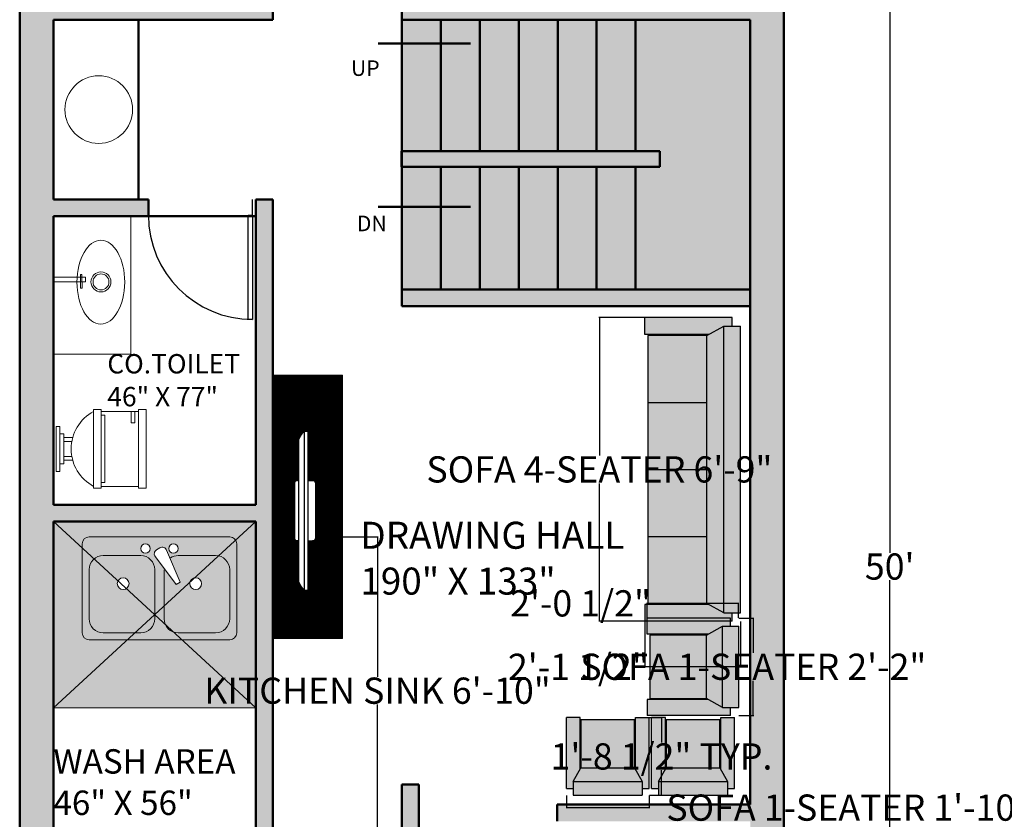
# Model space of a CAD drawing. Units: inches. Extents: x 679 to 1269, y 101 to 755.
# Tile 3 of 6: x 708 to 971, y 370 to 584. Entities that reach past the tile are written whole.
import ezdxf

# ---------------------------------------------------------------- set-up
doc = ezdxf.new("R2010")
doc.units = ezdxf.units.IN
doc.header["$MEASUREMENT"] = 0
for name, color, linetype, lineweight in [('A-ANNO-DIMS', 2, 'Continuous', 18), ('A-ANNO-TEXT', 7, 'Continuous', 25), ('A-AREA-IDEN', 7, 'Continuous', 25), ('A-DOOR', 4, 'Continuous', 25), ('A-FLOR-FIXT', 8, 'Continuous', 18), ('A-FLOR-PATT', 8, 'Continuous', 13), ('A-FURN', 32, 'Continuous', 18), ('A-FURN-PATT', 252, 'Continuous', 13), ('A-WALL', 7, 'Continuous', 50), ('A-WALL-PATT', 8, 'Continuous', 13)]:
    doc.layers.add(name, color=color, linetype=linetype, lineweight=lineweight)
doc.layers.add('furniture', color=32, linetype='Continuous')
doc.styles.add('ATT', font='TXT')
doc.styles.get("Standard").update_dxf_attribs({"font": 'arial.ttf'})
doc.dimstyles.get("Standard").update_dxf_attribs({"dimtxt": 7, "dimasz": 0.18, "dimexe": 0.18, "dimexo": 0.0625, "dimgap": 0.09, "dimtad": 0, "dimtih": 1, "dimtoh": 1, "dimzin": 0, "dimdsep": 46, "dimlunit": 3, "dimtxsty": 'Standard', "dimcen": 0.09, "dimadec": 0, "dimazin": 0, "dimtfac": 1, "dimtofl": 0, "dimtmove": 0, "dimatfit": 3, "dimfxl": 1, "dimtolj": 1, "dimtzin": 0, "dimarcsym": 0})

# ---------------------------------------------------------------- blocks, each defined once
blk = doc.blocks.new('*D2')
at = {"layer": 'A-ANNO-DIMS', "color": 0, "lineweight": -2, "transparency": 16777216}
for p, q in [((939.65, 737.73), (940.62, 737.73)), ((940.44, 737.55), (940.44, 441.39)), ((940.44, 137.91), (940.44, 434.07)), ((939.65, 137.73), (940.62, 137.73))]:
    blk.add_line(p, q, dxfattribs=at)
at = {"layer": 'A-ANNO-DIMS', "color": 0, "transparency": 16777216}
for points in [[(940.41, 737.55), (940.47, 737.55), (940.44, 737.73)], [(940.41, 137.91), (940.47, 137.91), (940.44, 137.73)]]:
    blk.add_solid(points, dxfattribs=at)
at = {"layer": 'Defpoints', "color": 0, "transparency": 16777216}
for p in [(939.59, 737.73), (939.59, 137.73), (940.44, 137.73)]:
    blk.add_point(p, dxfattribs=at)
at = {"layer": 'A-ANNO-DIMS', "color": 0, "transparency": 16777216, "insert": (940.44, 437.73), "char_height": 7, "attachment_point": 5}
blk.add_mtext("\\A1;50'", dxfattribs=at)
blk = doc.blocks.new('*U4')
for p, q in [((0, 0), (0, -6)), ((40, 0), (40, -6))]:
    blk.add_line(p, q)
blk.add_lwpolyline([(0, 0), (0, 40), (1.75, 40), (1.75, 0)], close=True)
blk.add_arc((0, 0), 40, 0, 90)
blk = doc.blocks.new('15PSNK10')
at = {"color": 0, "linetype": 'ByBlock'}
for p, q in [((0, 15), (0, -15)), ((20.5, 16.5), (1.5, 16.5)), ((7, 15), (17.5, 15)), ((22, -15), (22, 15)), ((4, 4), (4, 12)), ((20.5, 12), (20.5, 4)), ((2.37, -0.1), (2.77, 0.6)), ((10.18, -3.57), (4.27, 0.87)), ((17.5, 1), (7, 1)), ((2.88, -1.54), (9.68, -4.43)), ((7.04, -1), (17.5, -1)), ((4, -12), (4, -4)), ((9.68, -4.43), (10.18, -3.57)), ((20.5, -4), (20.5, -12)), ((1.5, -16.5), (20.5, -16.5)), ((17.5, -15), (7, -15))]:
    blk.add_line(p, q, dxfattribs=at)
for centre, radius in [((10, 7.75), 1.25), ((2.5, 3), 1), ((2.5, -3), 1), ((10, -7.75), 1.25)]:
    blk.add_circle(centre, radius, dxfattribs=at)
for centre, radius, start, end in [((1.5, 15), 1.5, 90, 180), ((7, 12), 3, 90, 180), ((17.5, 12), 3, 0, 90), ((20.5, 15), 1.5, 0, 90), ((7, 4), 3, 180, 270), ((17.5, 4), 3, 270, 0), ((3.63, 0.1), 1, 50.5377, 150), ((3.23, -0.6), 1, 150, 249.4623), ((17.5, -4), 3, 0, 90), ((7, -4), 3, 146.607, 180), ((7, -12), 3, 180, 270), ((17.5, -12), 3, 270, 0), ((1.5, -15), 1.5, 180, 270), ((20.5, -15), 1.5, 270, 0)]:
    blk.add_arc(centre, radius, start, end, dxfattribs=at)
at = {"color": 0, "linetype": 'ByBlock', "style": 'ATT'}
for tag, p, flags in [('ITEM', (0, -26), 3), ('ROOM_NUMBER', (0, -35), 1)]:
    blk.add_attdef(tag, p, '', height=6, dxfattribs=dict(at, flags=flags))
blk = doc.blocks.new('*U12')
for p, q in [((-10, 22), (-10, 12)), ((10, 12), (10, 22)), ((-10, 21), (-7, 21)), ((-7, 20), (-10, 20)), ((-7, 21), (-7, 20)), ((10.5, 12), (-10.5, 12)), ((-10.5, 10), (-10.5, 12)), ((9, 13), (-9, 13)), ((-9, 13), (-9, 12)), ((9, 12), (9, 13)), ((10.5, 12), (10.5, 10)), ((10.5, 10), (-10.5, 10)), ((-3, 4.4065), (-3, 2)), ((-2, 2), (-2, 4.1658)), ((2, 4.1658), (2, 2)), ((3, 2), (3, 4.4065)), ((4, 2), (-4, 2)), ((-4, 2), (-4, 1)), ((4, 1), (4, 2))]:
    blk.add_line(p, q)
for points in [[(10.5, 22), (10.5, 24), (-10.5, 24), (-10.5, 22)], [(6, 0), (6, 1), (-6, 1), (-6, 0)]]:
    blk.add_lwpolyline(points, close=True)
blk.add_arc((0, 15.3333), 11.3333, 208.0725, 331.9275)
blk = doc.blocks.new('FABRIC SOFA 4S')
at = {"layer": 'furniture'}
for p, q in [((3, 54), (34, 54)), ((3, 51), (3, 54)), ((34, 48), (34, 54)), ((0, -51), (0, 51)), ((6, 51), (0, 51)), ((6, -51), (6, 51)), ((12, 47.63), (6, 51)), ((11.14, 48), (34, 48)), ((33, 23.81), (12, 23.81)), ((33, 0), (12, 0)), ((33, -23.81), (12, -23.81)), ((6, -51), (12, -47.63)), ((11.54, -48), (34, -48)), ((34, -48), (34, -54)), ((6, -51), (0, -51)), ((3, -54), (3, -51)), ((3, -54), (34, -54))]:
    blk.add_line(p, q, dxfattribs=at)
blk.add_lwpolyline([(12, -47.63), (12, 47.63), (33, 47.63), (33, -47.63)], close=True, dxfattribs=at)
blk = doc.blocks.new('FABRIC SOFA 1S')
at = {"layer": 'furniture'}
for p, q in [((0, -15.12), (0, 15.12)), ((6, 15.12), (0, 15.12)), ((3, 18.12), (34, 18.12)), ((3, 15.12), (3, 18.12)), ((6, -15.12), (6, 15.12)), ((12, 11.75), (6, 15.12)), ((34, 12.12), (34, 18.12)), ((11.33, 12.12), (34, 12.12)), ((6, -15.12), (12, -11.75)), ((11.33, -12.12), (34, -12.12)), ((34, -12.12), (34, -18.12)), ((6, -15.12), (0, -15.12)), ((3, -18.12), (3, -15.12)), ((3, -18.12), (34, -18.12))]:
    blk.add_line(p, q, dxfattribs=at)
blk.add_lwpolyline([(12, -11.75), (12, 11.75), (33, 11.75), (33, -11.75)], close=True, dxfattribs=at)
blk = doc.blocks.new('PLASMA-LARGE')
at = {"layer": 'furniture'}
for p, q in [((-7.26, 0), (7.26, 0)), ((-21, -2.5), (21, -2.5)), ((-21, -2.5), (-21, -3.5)), ((-18.61, -1), (18.61, -1)), ((-8, -1), (-8, -0.74)), ((8, -1), (8, -0.74)), ((21, -2.5), (21, -3.5)), ((-21, -3.5), (21, -3.5)), ((-8, -3.5), (-8, -4.76)), ((8, -3.5), (8, -4.76)), ((-7.26, -5.5), (7.26, -5.5))]:
    blk.add_line(p, q, dxfattribs=at)
for centre, radius, start, end in [((-7.26, -0.74), 0.744, 90, 180), ((7.26, -0.74), 0.744, 0, 90), ((-13.97, -11.05), 11.07, 114.7602, 129.4175), ((13.97, -11.05), 11.07, 50.5825, 65.2398), ((-7.26, -4.76), 0.744, 180, 270), ((7.26, -4.76), 0.744, 270, 0)]:
    blk.add_arc(centre, radius, start, end, dxfattribs=at)
blk = doc.blocks.new('WASHBASIN')
for p, q in [((7.24, 9.62), (7.23, 13.28)), ((7.23, 13.28), (7.63, 13.28)), ((7.63, 13.28), (7.65, 9.63)), ((8.57, 12.49), (0, 12.49)), ((8.57, 11.25), (0, 11.25)), ((8.57, 11.25), (8.57, 12.49)), ((7.24, 9.62), (7.65, 9.63))]:
    blk.add_line(p, q)
for radius in [2.67, 2.13]:
    blk.add_circle((12.7, 11.27), radius)
at = {"extrusion": (0, 0, -1)}
blk.add_ellipse((12.66, 11.2), major_axis=(0.03, 11.2), ratio=0.56899, dxfattribs=at)
blk = doc.blocks.new('*D27')
at = {"layer": 'A-ANNO-DIMS', "color": 0, "lineweight": -2, "transparency": 16777216}
for p, q in [((854.14, 376.61), (854.14, 373.18)), ((876.23, 376.61), (876.23, 373.18)), ((854.32, 373.36), (876.05, 373.36)), ((876.23, 373.36), (876.41, 373.36))]:
    blk.add_line(p, q, dxfattribs=at)
at = {"layer": 'A-ANNO-DIMS', "color": 0, "transparency": 16777216}
for points in [[(854.32, 373.39), (854.32, 373.33), (854.14, 373.36)], [(876.05, 373.39), (876.05, 373.33), (876.23, 373.36)]]:
    blk.add_solid(points, dxfattribs=at)
at = {"layer": 'Defpoints', "color": 0, "transparency": 16777216}
for p in [(854.14, 376.67), (876.23, 376.67), (876.23, 373.36)]:
    blk.add_point(p, dxfattribs=at)
at = {"layer": 'A-ANNO-DIMS', "color": 0, "transparency": 16777216, "insert": (940.47, 373.36), "char_height": 7, "attachment_point": 5}
blk.add_mtext('\\A1;SOFA 1-SEATER 1\'-10" TYP.', dxfattribs=at)
blk = doc.blocks.new('*D28')
at = {"layer": 'A-ANNO-DIMS', "color": 0, "lineweight": -2, "transparency": 16777216}
for p, q in [((876.29, 397.39), (879.72, 397.39)), ((879.54, 397.21), (879.54, 390.74)), ((879.54, 376.85), (879.54, 383.32)), ((876.29, 376.67), (879.72, 376.67))]:
    blk.add_line(p, q, dxfattribs=at)
at = {"layer": 'A-ANNO-DIMS', "color": 0, "transparency": 16777216}
for points in [[(879.51, 397.21), (879.57, 397.21), (879.54, 397.39)], [(879.51, 376.85), (879.57, 376.85), (879.54, 376.67)]]:
    blk.add_solid(points, dxfattribs=at)
at = {"layer": 'Defpoints', "color": 0, "transparency": 16777216}
for p in [(876.23, 397.39), (879.54, 397.39), (876.23, 376.67)]:
    blk.add_point(p, dxfattribs=at)
at = {"layer": 'A-ANNO-DIMS', "color": 0, "transparency": 16777216, "insert": (879.54, 387.03), "char_height": 7, "attachment_point": 5}
blk.add_mtext('\\A1;1\'-8 1/2" TYP.', dxfattribs=at)
blk = doc.blocks.new('*D29')
at = {"layer": 'A-ANNO-DIMS', "color": 0, "lineweight": -2, "transparency": 16777216}
for p, q in [((900.19, 423.98), (904.22, 423.98)), ((904.04, 423.8), (904.04, 414.68)), ((904.04, 398.12), (904.04, 407.25)), ((900.19, 397.94), (904.22, 397.94))]:
    blk.add_line(p, q, dxfattribs=at)
at = {"layer": 'A-ANNO-DIMS', "color": 0, "transparency": 16777216}
for points in [[(904.01, 423.8), (904.07, 423.8), (904.04, 423.98)], [(904.01, 398.12), (904.07, 398.12), (904.04, 397.94)]]:
    blk.add_solid(points, dxfattribs=at)
at = {"layer": 'Defpoints', "color": 0, "transparency": 16777216}
for p in [(900.13, 423.98), (904.04, 423.98), (900.13, 397.94)]:
    blk.add_point(p, dxfattribs=at)
at = {"layer": 'A-ANNO-DIMS', "color": 0, "transparency": 16777216, "insert": (904.04, 410.96), "char_height": 7, "attachment_point": 5}
blk.add_mtext('\\A1;SOFA 1-SEATER 2\'-2"', dxfattribs=at)
blk = doc.blocks.new('*D30')
at = {"layer": 'A-ANNO-DIMS', "color": 0, "lineweight": -2, "transparency": 16777216}
for p, q in [((875.71, 427.89), (875.53, 427.89)), ((875.71, 424.05), (875.71, 428.07)), ((899.95, 427.89), (875.89, 427.89)), ((900.13, 424.05), (900.13, 428.07))]:
    blk.add_line(p, q, dxfattribs=at)
at = {"layer": 'A-ANNO-DIMS', "color": 0, "transparency": 16777216}
for points in [[(875.89, 427.92), (875.89, 427.86), (875.71, 427.89)], [(899.95, 427.92), (899.95, 427.86), (900.13, 427.89)]]:
    blk.add_solid(points, dxfattribs=at)
at = {"layer": 'Defpoints', "color": 0, "transparency": 16777216}
for p in [(875.71, 427.89), (875.71, 423.98), (900.13, 423.98)]:
    blk.add_point(p, dxfattribs=at)
at = {"layer": 'A-ANNO-DIMS', "color": 0, "transparency": 16777216, "insert": (857.92, 427.89), "char_height": 7, "attachment_point": 5}
blk.add_mtext('\\A1;2\'-0 1/2"', dxfattribs=at)
blk = doc.blocks.new('*D31')
at = {"layer": 'A-ANNO-DIMS', "color": 0, "lineweight": -2, "transparency": 16777216}
for p, q in [((834.08, 593.4), (834.08, 595.78)), ((834.26, 595.6), (849.02, 595.6)), ((849.2, 593.4), (849.2, 595.78)), ((849.2, 595.6), (849.38, 595.6))]:
    blk.add_line(p, q, dxfattribs=at)
at = {"layer": 'A-ANNO-DIMS', "color": 0, "transparency": 16777216}
for points in [[(834.26, 595.63), (834.26, 595.57), (834.08, 595.6)], [(849.02, 595.63), (849.02, 595.57), (849.2, 595.6)]]:
    blk.add_solid(points, dxfattribs=at)
at = {"layer": 'Defpoints', "color": 0, "transparency": 16777216}
for p in [(849.2, 595.6), (834.08, 593.34), (849.2, 593.34)]:
    blk.add_point(p, dxfattribs=at)
at = {"layer": 'A-ANNO-DIMS', "color": 0, "transparency": 16777216, "insert": (879.23, 595.6), "char_height": 7, "attachment_point": 5}
blk.add_mtext('\\A1;TV UNIT 1\'-3"', dxfattribs=at)
blk = doc.blocks.new('*D41')
at = {"layer": 'A-ANNO-DIMS', "color": 0, "lineweight": -2, "transparency": 16777216}
for p, q in [((875.06, 504.2), (862.78, 504.2)), ((862.96, 504.02), (862.96, 467.37)), ((862.96, 423.29), (862.96, 459.94)), ((875.06, 423.11), (862.78, 423.11))]:
    blk.add_line(p, q, dxfattribs=at)
at = {"layer": 'A-ANNO-DIMS', "color": 0, "transparency": 16777216}
for points in [[(862.93, 504.02), (862.99, 504.02), (862.96, 504.2)], [(862.93, 423.29), (862.99, 423.29), (862.96, 423.11)]]:
    blk.add_solid(points, dxfattribs=at)
at = {"layer": 'Defpoints', "color": 0, "transparency": 16777216}
for p in [(862.96, 504.2), (875.12, 504.2), (875.12, 423.11)]:
    blk.add_point(p, dxfattribs=at)
at = {"layer": 'A-ANNO-DIMS', "color": 0, "transparency": 16777216, "insert": (862.96, 463.66), "char_height": 7, "attachment_point": 5}
blk.add_mtext('\\A1;SOFA 4-SEATER 6\'-9"', dxfattribs=at)
blk = doc.blocks.new('*D42')
at = {"layer": 'A-ANNO-DIMS', "color": 0, "lineweight": -2, "transparency": 16777216}
for p, q in [((875.12, 423.05), (875.12, 410.77)), ((900.65, 423.05), (900.65, 410.77)), ((875.12, 410.95), (874.94, 410.95)), ((900.47, 410.95), (875.3, 410.95))]:
    blk.add_line(p, q, dxfattribs=at)
at = {"layer": 'A-ANNO-DIMS', "color": 0, "transparency": 16777216}
for points in [[(875.3, 410.98), (875.3, 410.92), (875.12, 410.95)], [(900.47, 410.98), (900.47, 410.92), (900.65, 410.95)]]:
    blk.add_solid(points, dxfattribs=at)
at = {"layer": 'Defpoints', "color": 0, "transparency": 16777216}
for p in [(875.12, 423.11), (900.65, 423.11), (875.12, 410.95)]:
    blk.add_point(p, dxfattribs=at)
at = {"layer": 'A-ANNO-DIMS', "color": 0, "transparency": 16777216, "insert": (857.33, 410.95), "char_height": 7, "attachment_point": 5}
blk.add_mtext('\\A1;2\'-1 1/2"', dxfattribs=at)
blk = doc.blocks.new('*D49')
at = {"layer": 'A-ANNO-DIMS', "color": 0, "lineweight": -2, "transparency": 16777216}
for p, q in [((791.46, 445.66), (803.9, 445.66)), ((803.72, 445.48), (803.72, 408.29)), ((803.72, 363.68), (803.72, 400.87)), ((791.46, 363.5), (803.9, 363.5))]:
    blk.add_line(p, q, dxfattribs=at)
at = {"layer": 'A-ANNO-DIMS', "color": 0, "transparency": 16777216}
for points in [[(803.69, 445.48), (803.75, 445.48), (803.72, 445.66)], [(803.69, 363.68), (803.75, 363.68), (803.72, 363.5)]]:
    blk.add_solid(points, dxfattribs=at)
at = {"layer": 'Defpoints', "color": 0, "transparency": 16777216}
for p in [(791.4, 445.66), (791.4, 363.5), (803.72, 363.5)]:
    blk.add_point(p, dxfattribs=at)
at = {"layer": 'A-ANNO-DIMS', "color": 0, "transparency": 16777216, "insert": (803.72, 404.58), "char_height": 7, "attachment_point": 5}
blk.add_mtext('\\A1;KITCHEN SINK 6\'-10"', dxfattribs=at)

msp = doc.modelspace()

# ---------------------------------------------------------------- hatches: boundary and pattern name
at = {"layer": 'A-FLOR-PATT'}
h = msp.add_hatch(dxfattribs=at)
h.set_pattern_fill('ANSI31', color=256)
h.paths.add_polyline_path([(1119.805, 251.542), (1104.539, 251.542), (1104.539, 181.227), (1119.805, 181.227)])
h.paths.add_polyline_path([(1111.468, 194.139), (1110.457, 194.139), (1110.457, 207.286), (1109.187, 207.286, -0.4142136), (1108.434, 208.038), (1108.434, 222.713, -0.4142136), (1109.187, 223.466), (1110.457, 223.466), (1110.457, 236.613), (1111.468, 236.613, -0.0640419), (1112.985, 234.194), (1112.985, 223.466), (1113.243, 223.466, -0.4142136), (1113.996, 222.713), (1113.996, 208.038, -0.4142136), (1113.243, 207.286), (1112.985, 207.286), (1112.985, 196.558, -0.0640419)], flags=16)
h.paths.add_polyline_path([(794.414, 488.811), (775.786, 488.811), (775.786, 449.729), (775.786, 418.496), (794.414, 418.496)])
h.paths.add_polyline_path([(785.134, 431.408), (784.123, 431.408, -0.0640419), (782.606, 433.827), (782.606, 444.555), (782.347, 444.555, -0.4142136), (781.595, 445.308), (781.595, 459.983, -0.4142136), (782.347, 460.736), (782.606, 460.736), (782.606, 471.463, -0.0640419), (784.123, 473.882), (785.134, 473.882), (785.134, 460.736), (786.404, 460.736, -0.4142136), (787.157, 459.983), (787.157, 445.308, -0.4142136), (786.404, 444.555), (785.134, 444.555)], flags=16)
at = {"layer": 'A-FURN-PATT'}
h = msp.add_hatch(color=256, dxfattribs=at)
h.dxf.hatch_style = 1
h.paths.add_polyline_path([(891.639, 499.41), (875.873, 499.41), (875.873, 481.533), (891.639, 481.533)], flags=17)
h.paths.add_polyline_path([(896.143, 501.944), (898.396, 501.944), (898.396, 504.196), (875.122, 504.196), (875.122, 499.692), (892.139, 499.692)])
h.paths.add_polyline_path([(896.143, 501.944), (891.639, 499.41), (891.639, 427.9), (896.143, 425.366)])
h.paths.add_polyline_path([(900.648, 501.944), (896.143, 501.944), (896.143, 425.366), (900.648, 425.366)])
h.paths.add_polyline_path([(891.639, 481.533), (875.873, 481.533), (875.873, 463.655), (891.639, 463.655)], flags=17)
h.paths.add_polyline_path([(891.639, 463.655), (875.873, 463.655), (875.873, 445.777), (891.639, 445.777)], flags=17)
h.paths.add_polyline_path([(891.639, 445.777), (875.873, 445.777), (875.873, 427.9), (891.639, 427.9)], flags=17)
h.paths.add_polyline_path([(891.639, 427.9), (875.873, 427.9), (875.873, 499.41), (891.639, 499.41), (891.639, 427.9), (896.143, 425.366), (898.396, 425.366), (898.396, 423.114), (897.977, 423.114), (897.977, 421.828), (900.132, 421.828), (900.132, 400.1), (897.977, 400.1), (897.977, 397.945), (875.709, 397.945), (875.709, 402.254), (891.991, 402.254), (891.512, 402.524), (876.428, 402.524), (876.428, 419.404), (891.512, 419.404), (891.991, 419.673), (875.709, 419.673), (875.709, 423.114), (875.122, 423.114), (875.122, 427.618), (892.139, 427.618)])
h = msp.add_hatch(color=256, dxfattribs=at)
h.dxf.hatch_style = 1
h.paths.add_polyline_path([(891.639, 499.41), (875.873, 499.41), (875.873, 481.533), (891.639, 481.533)])
h.paths.add_polyline_path([(891.639, 481.533), (875.873, 481.533), (875.873, 463.655), (891.639, 463.655)])
h.paths.add_polyline_path([(891.639, 463.655), (875.873, 463.655), (875.873, 445.777), (891.639, 445.777)])
h.paths.add_polyline_path([(891.639, 445.777), (875.873, 445.777), (875.873, 427.9), (891.639, 427.9)])
h = msp.add_hatch(color=256, dxfattribs=at)
h.dxf.hatch_style = 1
h.paths.add_polyline_path([(872.342, 396.782), (858.02, 396.782), (858.02, 383.984), (872.342, 383.984)])
h.paths.add_polyline_path([(857.792, 397.392), (854.135, 397.392), (854.135, 378.5), (855.963, 378.5), (855.963, 380.328), (857.792, 383.578)])
h.paths.add_polyline_path([(876.227, 397.392), (872.57, 397.392), (872.57, 383.578), (874.399, 380.328), (874.399, 378.5), (876.227, 378.5)])
h.paths.add_polyline_path([(872.342, 383.984), (858.02, 383.984), (855.963, 380.328), (874.399, 380.328)])
h.paths.add_polyline_path([(874.399, 380.328), (855.963, 380.328), (855.963, 376.671), (874.399, 376.671)])
h = msp.add_hatch(color=256, dxfattribs=at)
h.dxf.hatch_style = 1
h.paths.add_polyline_path([(895.107, 396.782), (880.785, 396.782), (880.785, 383.984), (895.107, 383.984)])
h.paths.add_polyline_path([(895.107, 383.984), (880.785, 383.984), (878.728, 380.328), (897.163, 380.328)])
h.paths.add_polyline_path([(897.163, 380.328), (878.728, 380.328), (878.728, 376.671), (897.163, 376.671)])
h.paths.add_polyline_path([(880.557, 397.392), (876.9, 397.392), (876.9, 378.5), (878.728, 378.5), (878.728, 380.328), (880.557, 383.578)])
h.paths.add_polyline_path([(898.992, 397.392), (895.335, 397.392), (895.335, 383.578), (897.163, 380.328), (897.163, 378.5), (898.992, 378.5)])
at = {"layer": 'A-WALL-PATT'}
h = msp.add_hatch(color=256, dxfattribs=at)
h.dxf.hatch_style = 1
h.paths.add_polyline_path([(775.786, 535.729), (771.286, 535.729), (771.286, 454.229), (717.214, 454.229), (717.214, 531.229), (742.559, 531.229), (742.559, 535.729), (717.214, 535.729), (717.214, 583.729), (775.786, 583.729), (775.786, 588.883), (775.786, 623.243), (775.786, 645.329), (771.286, 645.329), (771.286, 588.229), (717.214, 588.229), (717.214, 674.229), (734.589, 674.229), (734.589, 678.729), (717.214, 678.729), (717.214, 728.729), (903.214, 728.729), (903.214, 588.229), (810.214, 588.229), (810.214, 583.729), (903.214, 583.729), (903.214, 374.229), (851.714, 374.229), (851.714, 369.729), (903.214, 369.729), (903.214, 312.729), (856.214, 312.729), (856.214, 341.229), (851.714, 341.229), (851.714, 308.229), (903.214, 308.229), (903.214, 137.729), (912.214, 137.729), (912.214, 737.729), (708.214, 737.729), (708.214, 137.729), (717.214, 137.729), (717.214, 197.763), (776.196, 197.763), (776.196, 202.263), (717.214, 202.263), (717.214, 449.729), (771.286, 449.729), (771.286, 350.298), (775.786, 350.298), (775.786, 531.229)])
h = msp.add_hatch(color=256, dxfattribs=at)
h.dxf.hatch_style = 1
h.paths.add_polyline_path([(872.624, 583.729), (862.222, 583.729), (862.222, 548.661), (872.624, 548.661)])
h.paths.add_polyline_path([(862.222, 583.729), (851.821, 583.729), (851.821, 548.661), (862.222, 548.661)])
h.paths.add_polyline_path([(851.821, 583.729), (841.419, 583.729), (841.419, 548.661), (851.821, 548.661)])
h.paths.add_polyline_path([(841.419, 583.729), (831.017, 583.729), (831.017, 548.661), (841.419, 548.661)])
h.paths.add_polyline_path([(831.017, 583.729), (820.616, 583.729), (820.616, 548.661), (831.017, 548.661)])
h.paths.add_polyline_path([(820.616, 583.729), (810.214, 583.729), (810.214, 548.661), (820.616, 548.661)])
h = msp.add_hatch(color=256, dxfattribs=at)
h.dxf.hatch_style = 1
h.paths.add_polyline_path([(903.214, 583.729), (872.624, 583.729), (872.624, 548.661), (879.092, 548.661), (879.092, 544.406), (872.624, 544.406), (872.624, 511.729), (903.214, 511.729)])
h = msp.add_hatch(color=256, dxfattribs=at)
h.dxf.hatch_style = 1
h.paths.add_polyline_path([(810.214, 227.828), (741.495, 227.828), (741.495, 355.229), (717.214, 355.229), (717.214, 202.263), (810.214, 202.263)])
h.paths.add_polyline_path([(760.069, 222.258, -0.3244181), (762.516, 223.664), (788.753, 223.664, -0.4472035), (791.829, 221.27), (791.829, 207.648, -0.2614299), (789.688, 206.245), (762.516, 206.245, -0.3295457), (760.069, 207.722)], flags=16)
h.paths.add_polyline_path([(762.516, 221.27), (789.688, 221.27), (789.688, 208.13), (762.516, 208.13)], flags=0)
edge = h.paths.add_edge_path(flags=0)
edge.add_ellipse((783.813, 223.043), major_axis=(0.713, -0.02), ratio=0.3769734, start_angle=41.8657, end_angle=148.30827, ccw=False)
edge.add_line((783.879, 223.309), (790.017, 223.283))
edge.add_line((790.017, 223.283), (784.096, 223.283))
edge.add_ellipse((783.813, 223.043), major_axis=(0.713, -0.02), ratio=0.3769734, start_angle=346.43382, end_angle=401.8657, ccw=False)
edge.add_ellipse((783.805, 222.774), major_axis=(0.664, -0.043), ratio=0.4928397, start_angle=169.71962, end_angle=373.72858, ccw=False)
edge.add_ellipse((783.813, 223.043), major_axis=(0.713, -0.02), ratio=0.3769734, start_angle=148.30827, end_angle=192.13048, ccw=False)
h.paths.add_polyline_path([(772.808, 214.038, -1), (764.984, 214.038, -1)], flags=0)
h.paths.add_polyline_path([(766.816, 214.038, -1), (770.975, 214.038, -1)], flags=0)
h.paths.add_polyline_path([(767.671, 214.038, -1), (770.121, 214.038, -1)], flags=0)
edge = h.paths.add_edge_path(flags=0)
edge.add_ellipse((768.035, 222.547), major_axis=(0.664, -0.043), ratio=0.4928397, start_angle=165.08046, end_angle=377.66995, ccw=False)
edge.add_ellipse((768.056, 222.874), major_axis=(0.713, -0.02), ratio=0.3769734, start_angle=342.91014, end_angle=554.30055, ccw=False)
h.paths.add_polyline_path([(769.403, 214.038, -1), (768.389, 214.038, -1)], flags=0)
h.paths.add_polyline_path([(787.721, 214.038, -1), (779.897, 214.038, -1)], flags=0)
h.paths.add_polyline_path([(781.729, 214.038, -1), (785.889, 214.038, -1)], flags=0)
h.paths.add_polyline_path([(782.584, 214.038, -1), (785.034, 214.038, -1)], flags=0)
h.paths.add_polyline_path([(718.284, 266.795), (718.284, 299.81), (736.853, 299.81), (736.853, 266.795)], flags=16)
h.paths.add_polyline_path([(784.316, 214.038, -1), (783.302, 214.038, -1)], flags=0)
edge = h.paths.add_edge_path(flags=0)
edge.add_ellipse((729.652, 284.027), major_axis=(0.028, 10.061), ratio=0.5689904, start_angle=89.77279, end_angle=78.681, ccw=False)
edge.add_ellipse((729.652, 284.027), major_axis=(0.028, 10.061), ratio=0.5689904, start_angle=78.681, end_angle=89.77279, ccw=False)
h.paths.add_polyline_path([(727.295, 284.083, -1), (732.089, 284.083, -1)], flags=0)
h.paths.add_polyline_path([(727.778, 284.083, -1), (731.606, 284.083, -1)], flags=0)
h.paths.add_polyline_path([(725.151, 282.611), (724.79, 282.604), (724.774, 285.892), (725.136, 285.894), (725.139, 285.181), (725.979, 285.181), (725.984, 284.066), (725.144, 284.066)], flags=0)
h.paths.add_polyline_path([(719.385, 333.571), (719.385, 353.397), (736.221, 353.397), (736.221, 334.653), (740.278, 340.163), (741.05, 339.707), (736.221, 333.571)], flags=16)
h.paths.add_polyline_path([(751.548, 418.161), (736.952, 418.161), (717.214, 400.013), (771.286, 400.013)])
h.paths.add_polyline_path([(736.952, 418.161), (726.768, 418.161, -0.4142136), (724.894, 420.036), (724.894, 442.668), (717.214, 449.729), (717.214, 400.013)])
h.paths.add_polyline_path([(771.286, 449.729), (765.869, 444.749, -0.1362876), (766.138, 443.782), (766.138, 420.036, -0.4142136), (764.263, 418.161), (751.548, 418.161), (771.286, 400.013)])
h.paths.add_polyline_path([(771.286, 449.729), (717.214, 449.729), (724.894, 442.668), (724.894, 443.782, -0.4142136), (726.768, 445.657), (764.263, 445.657, -0.2630748), (765.869, 444.749)])
h.paths.add_polyline_path([(797.166, 526.216), (807.611, 526.216), (807.611, 532.439), (797.166, 532.439)], flags=9)
h.paths.add_polyline_path([(795.576, 567.589), (805.736, 567.589), (805.736, 573.918), (795.576, 573.918)], flags=9)
h.paths.add_polyline_path([(858.791, 331.287), (904.364, 331.287), (904.364, 342.335), (858.791, 342.335)], flags=9)
h.paths.add_polyline_path([(858.766, 343.502), (896.669, 343.502), (896.669, 354.698), (858.766, 354.698)], flags=9)
h.paths.add_polyline_path([(797.309, 428.261), (854.093, 428.261), (854.093, 439.317), (797.309, 439.317)], flags=9)
h.paths.add_polyline_path([(797.287, 440.484), (877.723, 440.484), (877.723, 451.673), (797.287, 451.673)], flags=9)
h.paths.add_polyline_path([(715.552, 369.625), (756.685, 369.625), (756.685, 379.597), (715.552, 379.597)], flags=9)
h.paths.add_polyline_path([(715.531, 380.652), (773.487, 380.652), (773.487, 390.75), (715.531, 390.75)], flags=9)
h.paths.add_polyline_path([(814.122, 344.048), (852.566, 344.048), (852.566, 355.244), (814.122, 355.244)], flags=9)
h.paths.add_polyline_path([(749.801, 259.222), (806.583, 259.222), (806.583, 270.27), (749.801, 270.27)], flags=25)
h.paths.add_polyline_path([(749.778, 271.439), (797.735, 271.439), (797.735, 282.627), (749.778, 282.627)], flags=25)
h.paths.add_polyline_path([(730.28, 479.1), (762.944, 479.1), (762.944, 487.018), (730.28, 487.018)], flags=9)
h.paths.add_polyline_path([(730.263, 487.855), (771.058, 487.855), (771.058, 495.879), (730.263, 495.879)], flags=9)
h = msp.add_hatch(color=256, dxfattribs=at)
h.dxf.hatch_style = 1
h.paths.add_polyline_path([(879.092, 548.661), (810.214, 548.661), (810.214, 544.406), (879.092, 544.406)])
h = msp.add_hatch(color=256, dxfattribs=at)
h.dxf.hatch_style = 1
h.paths.add_polyline_path([(872.624, 544.406), (862.222, 544.406), (862.222, 511.729), (872.624, 511.729)])
h.paths.add_polyline_path([(862.222, 544.406), (851.821, 544.406), (851.821, 511.729), (862.222, 511.729)])
h.paths.add_polyline_path([(851.821, 544.406), (841.419, 544.406), (841.419, 511.729), (851.821, 511.729)])
h.paths.add_polyline_path([(841.419, 544.406), (831.017, 544.406), (831.017, 511.729), (841.419, 511.729)])
h.paths.add_polyline_path([(831.017, 544.406), (820.616, 544.406), (820.616, 511.729), (831.017, 511.729)])
h.paths.add_polyline_path([(820.616, 544.406), (810.214, 544.406), (810.214, 511.729), (820.616, 511.729)])
h = msp.add_hatch(color=256, dxfattribs=at)
h.dxf.hatch_style = 1
h.paths.add_polyline_path([(903.214, 511.729), (810.214, 511.729), (810.214, 507.229), (903.214, 507.229)])
h.paths.add_polyline_path([(881.964, 303.729), (903.214, 303.729), (903.214, 308.229), (877.464, 308.229), (877.464, 137.729), (903.214, 137.729), (903.214, 142.229), (881.964, 142.229), (881.964, 151.229)])
h.paths.add_polyline_path([(814.714, 379.54), (810.214, 379.54), (810.214, 197.763), (814.714, 197.763)])
h = msp.add_hatch(color=256, dxfattribs=at)
h.dxf.hatch_style = 1
h.paths.add_polyline_path([(744.266, 436.908, 0.4142136), (740.516, 440.658), (730.518, 440.658, 0.4142136), (726.768, 436.908), (726.768, 423.785, 0.4142136), (730.518, 420.036), (740.516, 420.036, 0.4142136), (744.266, 423.785)], flags=0)
h.paths.add_polyline_path([(734.267, 433.159, -1), (737.392, 433.159, -1)], flags=0)
h.paths.add_polyline_path([(766.138, 443.782, 0.4142136), (764.263, 445.657), (726.768, 445.657, 0.4142136), (724.894, 443.782), (724.894, 420.036, 0.4142136), (726.768, 418.161), (764.263, 418.161, 0.4142136), (766.138, 420.036)])
h.paths.add_polyline_path([(753.64, 433.159, -1), (756.764, 433.159, -1)], flags=16)
h.paths.add_polyline_path([(751.056, 433.561), (749.974, 432.936), (744.427, 440.32, -0.4631975), (744.766, 442.197), (745.638, 442.7, -0.4637074), (747.435, 442.057)], flags=16)
h.paths.add_polyline_path([(744.266, 423.785, -0.4142136), (740.516, 420.036), (730.518, 420.036, -0.4142136), (726.768, 423.785), (726.768, 436.908, -0.4142136), (730.518, 440.658), (740.516, 440.658, -0.4142136), (744.266, 436.908)], flags=16)
h.paths.add_polyline_path([(748.015, 442.533, -1), (750.515, 442.533, -1)], flags=16)
h.paths.add_polyline_path([(740.516, 442.533, -1), (743.016, 442.533, -1)], flags=16)
h = msp.add_hatch(color=256, dxfattribs=at)
h.dxf.hatch_style = 1
h.paths.add_polyline_path([(744.266, 436.908, 0.4142136), (740.516, 440.658), (730.518, 440.658, 0.4142136), (726.768, 436.908), (726.768, 423.785, 0.4142136), (730.518, 420.036), (740.516, 420.036, 0.4142136), (744.266, 423.785)])
h.paths.add_polyline_path([(734.267, 433.159, -1), (737.392, 433.159, -1)], flags=16)

# ---------------------------------------------------------------- linework, layer by layer
at = {"layer": 'A-FLOR-FIXT'}
for p, q in [((717.214, 531.229), (737.891, 531.229)), ((717.214, 494.465), (717.214, 531.229)), ((737.891, 531.229), (737.891, 494.465)), ((737.891, 494.465), (717.214, 494.465)), ((717.214, 400.013), (771.286, 449.729)), ((771.286, 400.013), (717.214, 449.729)), ((771.286, 400.013), (717.214, 400.013))]:
    msp.add_line(p, q, dxfattribs=at)
at = {"layer": 'A-FURN'}
for p, q in [((775.786, 488.811), (794.414, 488.811)), ((794.414, 488.811), (794.414, 418.496)), ((794.414, 418.496), (775.786, 418.496))]:
    msp.add_line(p, q, dxfattribs=at)
msp.add_circle((729.324, 559.729), 9.024, dxfattribs=at)
at = {"layer": 'A-WALL'}
for p, q in [((708.214, 137.729), (708.214, 737.729)), ((912.214, 737.729), (912.214, 137.729)), ((775.786, 583.729), (775.786, 645.329)), ((775.786, 583.729), (775.786, 645.329)), ((775.786, 623.243), (775.786, 583.729)), ((810.214, 583.729), (810.214, 588.229)), ((717.214, 583.729), (775.786, 583.729)), ((717.214, 535.729), (717.214, 583.729)), ((717.214, 535.729), (717.214, 583.729)), ((739.953, 583.729), (739.953, 535.729)), ((810.214, 583.729), (903.214, 583.729)), ((810.214, 583.729), (810.214, 511.729)), ((820.616, 583.729), (820.616, 548.661)), ((831.017, 583.729), (831.017, 548.661)), ((841.419, 583.729), (841.419, 548.661)), ((851.821, 583.729), (851.821, 548.661)), ((862.222, 583.729), (862.222, 548.661)), ((872.624, 583.729), (872.624, 548.661)), ((903.214, 583.729), (903.214, 374.229)), ((803.869, 577.34), (828.541, 577.34)), ((810.145, 548.661), (879.092, 548.661)), ((810.145, 544.406), (810.145, 548.661)), ((879.092, 548.661), (879.092, 544.406)), ((879.092, 544.406), (810.145, 544.406)), ((820.616, 544.406), (820.616, 511.729)), ((831.017, 544.406), (831.017, 511.729)), ((841.419, 544.406), (841.419, 511.729)), ((851.821, 544.406), (851.821, 511.729)), ((862.222, 544.406), (862.222, 511.729)), ((872.624, 544.406), (872.624, 511.729)), ((717.214, 535.729), (742.559, 535.729)), ((742.559, 535.729), (742.559, 531.554)), ((771.286, 454.229), (771.286, 535.729)), ((771.286, 535.729), (775.786, 535.729)), ((775.786, 449.729), (775.786, 535.729)), ((803.869, 533.743), (828.541, 533.743)), ((717.214, 509.729), (717.214, 531.229)), ((717.214, 531.229), (771.286, 531.229)), ((717.214, 454.229), (717.214, 531.229)), ((771.286, 454.229), (771.286, 531.229)), ((775.786, 350.298), (775.786, 531.229)), ((810.214, 511.729), (903.214, 511.729)), ((810.214, 511.729), (810.214, 507.229)), ((810.214, 507.229), (903.214, 507.229)), ((717.214, 454.229), (771.286, 454.229)), ((717.214, 449.729), (771.286, 449.729)), ((717.214, 202.263), (717.214, 449.729)), ((771.286, 350.298), (771.286, 449.729)), ((810.214, 379.54), (814.714, 379.54)), ((810.214, 197.763), (810.214, 379.54)), ((814.714, 137.729), (814.714, 379.54)), ((851.714, 374.229), (903.214, 374.229)), ((851.714, 374.229), (851.714, 369.729))]:
    msp.add_line(p, q, dxfattribs=at)

# ---------------------------------------------------------------- block references
at = {"layer": 'A-DOOR', "xscale": 0.8589852122862605, "yscale": 0.8589852122862605, "zscale": 0.8589852122862605}
msp.add_blockref('*U4', (775.786, 588.883), dxfattribs=at)
at = {"layer": 'A-DOOR', "xscale": 0.6958591214377364, "yscale": 0.6958591214377364, "zscale": 0.6958591214377364, "rotation": 180}
msp.add_blockref('*U4', (770.394, 531.554), dxfattribs=at)
at = {"layer": 'A-FLOR-FIXT'}
msp.add_blockref('WASHBASIN', (717.214, 502.451), dxfattribs=at)
at = {"layer": 'A-FLOR-FIXT', "rotation": 269.9999999999999}
msp.add_blockref('*U12', (717.955, 469.134), dxfattribs=at)
at = {"layer": 'A-FLOR-FIXT', "xscale": -1.249815573710304, "yscale": 1.249815573710304, "zscale": 1.249815573710304, "rotation": 90}
msp.add_blockref('15PSNK10', (745.516, 445.657), dxfattribs=at)
at = {"layer": 'A-FURN'}
for name, p, xscale, yscale, zscale in [('FABRIC SOFA 4S', (900.648, 463.655), -0.7507637528364199, 0.7507637528364199, 0.7507637528364199), ('FABRIC SOFA 1S', (900.132, 410.964), -0.7182990901146336, 0.7182990901146336, 0.7182990901146336)]:
    msp.add_blockref(name, p, dxfattribs=dict(at, xscale=xscale, yscale=yscale, zscale=zscale))
for name, p, xscale, yscale, zscale, rotation in [('PLASMA-LARGE', (781.595, 452.645), -1.011294184530666, 1.011294184530666, 1.011294184530666, 90), ('FABRIC SOFA 1S', (865.181, 376.671), -0.6094251026746103, 0.6094251026746103, 0.6094251026746103, 270), ('FABRIC SOFA 1S', (887.946, 376.671), -0.6094251026746103, 0.6094251026746103, 0.6094251026746103, 270)]:
    msp.add_blockref(name, p, dxfattribs=dict(at, xscale=xscale, yscale=yscale, zscale=zscale, rotation=rotation))

# ---------------------------------------------------------------- texts
at = {"layer": 'A-ANNO-TEXT'}
for s, p in [('UP', (796.631, 568.715)), ('DN', (798.203, 527.253))]:
    msp.add_text(s, height=4.1487, dxfattribs=at).set_placement(p)
at = {"layer": 'A-AREA-IDEN'}
for s, height, p in [('CO.TOILET', 5.1697, (731.6, 489.28)), ('46" X 77"', 5.1697, (731.6, 480.507)), ('DRAWING HALL', 7.21303, (799.152, 442.472)), ('190" X 133"', 7.21303, (799.152, 430.232)), ('WASH AREA', 6.5101, (717.214, 382.446)), ('46" X 56"', 6.5101, (717.214, 371.398))]:
    msp.add_text(s, height=height, dxfattribs=at).set_placement(p)

# ---------------------------------------------------------------- dimensions: what is measured, and where the dimension line sits
at = {"layer": 'A-ANNO-DIMS'}
for base, p1, p2, angle, override, picture, middle in [((940.437, 137.729), (939.586, 737.729), (939.586, 137.729), 90, {"dimclrd": 0, "dimclre": 0, "dimclrt": 0}, '*D2', (940.437, 437.729)), ((875.709, 427.889), (900.132, 423.983), (875.709, 423.983), 180, {"dimdec": 1, "dimrnd": 0, "dimzin": 1, "dimlunit": 4, "dimfrac": 2}, '*D30', (857.92, 427.889)), ((875.122, 410.951), (900.648, 423.114), (875.122, 423.114), 180, {"dimdec": 1, "dimrnd": 0, "dimzin": 1, "dimlunit": 4, "dimfrac": 2}, '*D42', (857.333, 410.951))]:
    dim = msp.add_linear_dim(base=base, p1=p1, p2=p2, angle=angle, dimstyle='Standard', override=override, dxfattribs=at)
    dim.commit()
    dim.dimension.update_dxf_attribs({"geometry": picture, "text_midpoint": middle})
for base, p1, p2, text, picture, middle in [((849.196, 595.603), (834.08, 593.336), (849.196, 593.336), 'TV UNIT <>', '*D31', (879.231, 595.603)), ((876.227, 373.358), (854.135, 376.671), (876.227, 376.671), 'SOFA 1-SEATER <> TYP.', '*D27', (940.473, 373.358))]:
    dim = msp.add_linear_dim(base=base, p1=p1, p2=p2, text=text, dimstyle='Standard', override={"dimdec": 1, "dimrnd": 0, "dimzin": 1, "dimlunit": 4, "dimfrac": 2}, dxfattribs=at)
    dim.commit()
    dim.dimension.update_dxf_attribs({"geometry": picture, "text_midpoint": middle})
for base, p1, p2, angle, text, picture, middle in [((862.96, 504.196), (875.122, 423.114), (875.122, 504.196), 90, 'SOFA 4-SEATER <>', '*D41', (862.96, 463.655)), ((803.723, 363.496), (791.399, 445.657), (791.399, 363.496), 270, 'KITCHEN SINK <>', '*D49', (803.723, 404.577)), ((904.037, 423.983), (900.132, 397.945), (900.132, 423.983), 90, 'SOFA 1-SEATER <>', '*D29', (904.037, 410.964)), ((879.541, 397.392), (876.227, 376.671), (876.227, 397.392), 90, '<> TYP.', '*D28', (879.541, 387.032))]:
    dim = msp.add_linear_dim(base=base, p1=p1, p2=p2, angle=angle, text=text, dimstyle='Standard', override={"dimdec": 1, "dimrnd": 0, "dimzin": 1, "dimlunit": 4, "dimfrac": 2}, dxfattribs=at)
    dim.commit()
    dim.dimension.update_dxf_attribs({"geometry": picture, "text_midpoint": middle})

doc.saveas('drawing.dxf')
